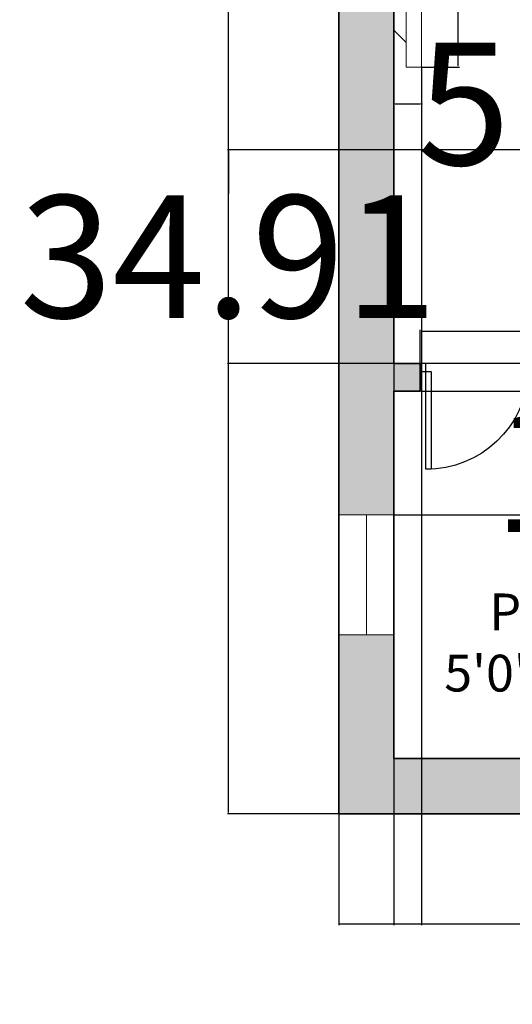
# Model space of a CAD drawing. Units: inches. Extents: x 305 to 776, y 38 to 479.
# Tile 1 of 14: x 339 to 419, y 38 to 199. Entities that reach past the tile are written whole.
import ezdxf

# ---------------------------------------------------------------- set-up
doc = ezdxf.new("R2010")
doc.units = ezdxf.units.IN
doc.header["$MEASUREMENT"] = 0
for name, color, linetype, lineweight in [('A-ANNO-DIMS', 2, 'Continuous', 18), ('A-AREA-IDEN', 7, 'Continuous', 18), ('A-DOOR', 4, 'Continuous', 25), ('A-EQPM', 8, 'Continuous', 18), ('A-GLAZ', 4, 'Continuous', 20), ('A-WALL', 7, 'Continuous', 35), ('A-WALL-PATT', 252, 'Continuous', 13)]:
    doc.layers.add(name, color=color, linetype=linetype, lineweight=lineweight)
doc.styles.get("Standard").update_dxf_attribs({"font": 'arial.ttf'})
doc.dimstyles.get("Standard").update_dxf_attribs({"dimtxt": 20, "dimasz": 0.18, "dimexe": 0.18, "dimexo": 0.0625, "dimgap": 0.09, "dimtad": 0, "dimtih": 1, "dimtoh": 1, "dimdec": 4, "dimzin": 0, "dimdsep": 46, "dimtxsty": 'Standard', "dimcen": 0.09, "dimadec": 0, "dimazin": 0, "dimtfac": 1, "dimtdec": 4, "dimtofl": 0, "dimtmove": 0, "dimatfit": 3, "dimfxl": 1, "dimtolj": 1, "dimtzin": 0, "dimarcsym": 0})

# ---------------------------------------------------------------- blocks, each defined once
blk = doc.blocks.new('W1')
blk.add_line((867.01, 338.44), (847.41, 338.44))
blk.add_lwpolyline([(847.41, 333.94), (867.01, 333.94), (867.01, 342.94), (847.41, 342.94)], close=True)
blk = doc.blocks.new('TV')
for p, q in [((722.63, 295.63), (720.13, 295.63)), ((720.13, 295.63), (720.13, 255.63)), ((722.63, 255.63), (722.63, 295.63)), ((720.13, 291.63), (718.13, 289.63)), ((718.13, 289.63), (718.13, 261.63)), ((720.13, 259.63), (718.13, 261.63)), ((720.13, 255.63), (722.63, 255.63))]:
    blk.add_line(p, q)
blk = doc.blocks.new('A$C16FA5A5B')
for p, q in [((50, 487.5), (25, 487.5)), ((25, 487.5), (25, 37.5)), ((50, 37.5), (50, 487.5)), ((950, 37.5), (950, 487.5)), ((950, 487.5), (975, 487.5)), ((975, 487.5), (975, 37.5)), ((0, 0), (0, 37.5)), ((0, 37.5), (25, 37.5)), ((25, 0), (0, 0)), ((25, 37.5), (25, 0)), ((25, 37.5), (50, 37.5)), ((975, 37.5), (950, 37.5)), ((975, 37.5), (975, 0)), ((1000, 37.5), (975, 37.5)), ((975, 0), (1000, 0)), ((1000, 0), (1000, 37.5))]:
    blk.add_line(p, q)
for centre, start, end in [((28.6, 15.6), 2.662, 90.4344), ((971.4, 15.6), 89.5656, 177.338)]:
    blk.add_arc(centre, 471.9, start, end)
blk = doc.blocks.new('*D21')
at = {"layer": 'A-ANNO-DIMS', "color": 0, "lineweight": -2, "transparency": 16777216}
for p, q in [((403.93, 142.94), (403.93, 148.37)), ((404.11, 148.19), (439.15, 148.19)), ((439.33, 142.94), (439.33, 148.37)), ((439.33, 148.19), (439.51, 148.19))]:
    blk.add_line(p, q, dxfattribs=at)
at = {"layer": 'A-ANNO-DIMS', "color": 0, "transparency": 16777216}
for points in [[(404.11, 148.22), (404.11, 148.16), (403.93, 148.19)], [(439.15, 148.22), (439.15, 148.16), (439.33, 148.19)]]:
    blk.add_solid(points, dxfattribs=at)
at = {"layer": 'Defpoints', "color": 0, "transparency": 16777216}
for p in [(439.33, 148.19), (403.93, 142.88), (439.33, 142.88)]:
    blk.add_point(p, dxfattribs=at)
at = {"layer": 'A-ANNO-DIMS', "color": 0, "transparency": 16777216, "insert": (560.63, 148.19), "char_height": 20, "attachment_point": 5}
blk.add_mtext('\\A1;DOUBLE DOOR 35', dxfattribs=at)
blk = doc.blocks.new('*D22')
at = {"layer": 'A-ANNO-DIMS', "color": 0, "lineweight": -2, "transparency": 16777216}
for p, q in [((439.4, 142.88), (444.82, 142.88)), ((444.64, 142.7), (444.64, 125.74)), ((439.4, 125.56), (444.82, 125.56)), ((444.64, 125.56), (444.64, 125.38)), ((444.64, 125.38), (444.46, 125.38))]:
    blk.add_line(p, q, dxfattribs=at)
at = {"layer": 'A-ANNO-DIMS', "color": 0, "transparency": 16777216}
for points in [[(444.61, 142.7), (444.67, 142.7), (444.64, 142.88)], [(444.61, 125.74), (444.67, 125.74), (444.64, 125.56)]]:
    blk.add_solid(points, dxfattribs=at)
at = {"layer": 'Defpoints', "color": 0, "transparency": 16777216}
for p in [(439.33, 142.88), (439.33, 125.56), (444.64, 125.56)]:
    blk.add_point(p, dxfattribs=at)
at = {"layer": 'A-ANNO-DIMS', "color": 0, "transparency": 16777216, "insert": (430.99, 125.38), "char_height": 20, "attachment_point": 5}
blk.add_mtext('\\A1;17', dxfattribs=at)
blk = doc.blocks.new('*D37')
at = {"layer": 'A-ANNO-DIMS', "color": 0, "lineweight": -2, "transparency": 16777216}
for p, q in [((476.35, 237.03), (483.22, 237.03)), ((483.04, 236.85), (483.04, 224.94)), ((483.04, 192.15), (483.04, 204.06)), ((476.35, 191.97), (483.22, 191.97))]:
    blk.add_line(p, q, dxfattribs=at)
at = {"layer": 'A-ANNO-DIMS', "color": 0, "transparency": 16777216}
for points in [[(483.01, 236.85), (483.07, 236.85), (483.04, 237.03)], [(483.01, 192.15), (483.07, 192.15), (483.04, 191.97)]]:
    blk.add_solid(points, dxfattribs=at)
at = {"layer": 'Defpoints', "color": 0, "transparency": 16777216}
for p in [(476.28, 237.03), (483.04, 237.03), (476.28, 191.97)]:
    blk.add_point(p, dxfattribs=at)
at = {"layer": 'A-ANNO-DIMS', "color": 0, "transparency": 16777216, "insert": (483.04, 214.5), "char_height": 20, "attachment_point": 5}
blk.add_mtext('\\A1;COFFEE TABLE 45', dxfattribs=at)
blk = doc.blocks.new('*D39')
at = {"layer": 'A-ANNO-DIMS', "color": 0, "lineweight": -2, "transparency": 16777216}
for p, q in [((404.2, 231.29), (410.31, 231.29)), ((410.13, 231.11), (410.13, 221.59)), ((410.13, 191.47), (410.13, 200.99)), ((404.2, 191.29), (410.31, 191.29))]:
    blk.add_line(p, q, dxfattribs=at)
at = {"layer": 'A-ANNO-DIMS', "color": 0, "transparency": 16777216}
for points in [[(410.1, 231.11), (410.16, 231.11), (410.13, 231.29)], [(410.1, 191.47), (410.16, 191.47), (410.13, 191.29)]]:
    blk.add_solid(points, dxfattribs=at)
at = {"layer": 'Defpoints', "color": 0, "transparency": 16777216}
for p in [(404.13, 231.29), (410.13, 231.29), (404.13, 191.29)]:
    blk.add_point(p, dxfattribs=at)
at = {"layer": 'A-ANNO-DIMS', "color": 0, "transparency": 16777216, "insert": (410.13, 211.29), "char_height": 20, "attachment_point": 5}
blk.add_mtext('\\A1;TV 40', dxfattribs=at)
blk = doc.blocks.new('*D40')
at = {"layer": 'A-ANNO-DIMS', "color": 0, "lineweight": -2, "transparency": 16777216}
for p, q in [((399.63, 191.23), (399.63, 185.11)), ((404.13, 191.23), (404.13, 185.11)), ((399.81, 185.29), (403.95, 185.29)), ((404.13, 185.29), (404.31, 185.29))]:
    blk.add_line(p, q, dxfattribs=at)
at = {"layer": 'A-ANNO-DIMS', "color": 0, "transparency": 16777216}
for points in [[(399.81, 185.32), (399.81, 185.26), (399.63, 185.29)], [(403.95, 185.32), (403.95, 185.26), (404.13, 185.29)]]:
    blk.add_solid(points, dxfattribs=at)
at = {"layer": 'Defpoints', "color": 0, "transparency": 16777216}
for p in [(399.63, 191.29), (404.13, 191.29), (404.13, 185.29)]:
    blk.add_point(p, dxfattribs=at)
at = {"layer": 'A-ANNO-DIMS', "color": 0, "transparency": 16777216, "insert": (411.03, 185.29), "char_height": 20, "attachment_point": 5}
blk.add_mtext('\\A1;5', dxfattribs=at)
blk = doc.blocks.new('*D45')
at = {"layer": 'A-ANNO-DIMS', "color": 0, "lineweight": -2, "transparency": 16777216}
for p, q in [((390.63, 69.32), (390.63, 51.2)), ((630.63, 69.32), (630.63, 51.2)), ((390.81, 51.38), (488.31, 51.38)), ((630.45, 51.38), (532.95, 51.38))]:
    blk.add_line(p, q, dxfattribs=at)
at = {"layer": 'A-ANNO-DIMS', "color": 0, "transparency": 16777216}
for points in [[(390.81, 51.41), (390.81, 51.35), (390.63, 51.38)], [(630.45, 51.41), (630.45, 51.35), (630.63, 51.38)]]:
    blk.add_solid(points, dxfattribs=at)
at = {"layer": 'Defpoints', "color": 0, "transparency": 16777216}
for p in [(390.63, 69.38), (630.63, 69.38), (630.63, 51.38)]:
    blk.add_point(p, dxfattribs=at)
at = {"layer": 'A-ANNO-DIMS', "color": 0, "transparency": 16777216, "insert": (510.63, 51.38), "char_height": 20, "attachment_point": 5}
blk.add_mtext('\\A1;240', dxfattribs=at)
blk = doc.blocks.new('*D46')
at = {"layer": 'A-ANNO-DIMS', "color": 0, "lineweight": -2, "transparency": 16777216}
for p, q in [((390.57, 429.38), (372.45, 429.38)), ((372.63, 429.2), (372.63, 259.69)), ((372.63, 69.56), (372.63, 239.07)), ((390.57, 69.38), (372.45, 69.38))]:
    blk.add_line(p, q, dxfattribs=at)
at = {"layer": 'A-ANNO-DIMS', "color": 0, "transparency": 16777216}
for points in [[(372.6, 429.2), (372.66, 429.2), (372.63, 429.38)], [(372.6, 69.56), (372.66, 69.56), (372.63, 69.38)]]:
    blk.add_solid(points, dxfattribs=at)
at = {"layer": 'Defpoints', "color": 0, "transparency": 16777216}
for p in [(372.63, 429.38), (390.63, 429.38), (390.63, 69.38)]:
    blk.add_point(p, dxfattribs=at)
at = {"layer": 'A-ANNO-DIMS', "color": 0, "transparency": 16777216, "insert": (372.63, 249.38), "char_height": 20, "attachment_point": 5}
blk.add_mtext('\\A1;360', dxfattribs=at)
blk = doc.blocks.new('*D48')
at = {"layer": 'A-ANNO-DIMS', "color": 0, "lineweight": -2, "transparency": 16777216}
for p, q in [((404, 138.38), (648.81, 138.38)), ((648.63, 138.38), (648.63, 138.56)), ((648.63, 138.56), (648.81, 138.56)), ((648.63, 118.36), (648.63, 138.2)), ((399.7, 118.18), (648.81, 118.18))]:
    blk.add_line(p, q, dxfattribs=at)
at = {"layer": 'A-ANNO-DIMS', "color": 0, "transparency": 16777216}
for points in [[(648.6, 138.2), (648.66, 138.2), (648.63, 138.38)], [(648.6, 118.36), (648.66, 118.36), (648.63, 118.18)]]:
    blk.add_solid(points, dxfattribs=at)
at = {"layer": 'Defpoints', "color": 0, "transparency": 16777216}
for p in [(403.93, 138.38), (648.63, 138.38), (399.63, 118.18)]:
    blk.add_point(p, dxfattribs=at)
at = {"layer": 'A-ANNO-DIMS', "color": 0, "transparency": 16777216, "insert": (674.95, 138.56), "char_height": 20, "attachment_point": 5}
blk.add_mtext('\\A1;20.2', dxfattribs=at)
blk = doc.blocks.new('*D62')
at = {"layer": 'A-ANNO-DIMS', "color": 0, "lineweight": -2, "transparency": 16777216}
for p, q in [((399.63, 336.32), (399.63, 51.2)), ((423.23, 336.32), (423.23, 51.2)), ((399.81, 51.38), (423.05, 51.38)), ((423.23, 51.38), (423.41, 51.38))]:
    blk.add_line(p, q, dxfattribs=at)
at = {"layer": 'A-ANNO-DIMS', "color": 0, "transparency": 16777216}
for points in [[(399.81, 51.41), (399.81, 51.35), (399.63, 51.38)], [(423.05, 51.41), (423.05, 51.35), (423.23, 51.38)]]:
    blk.add_solid(points, dxfattribs=at)
at = {"layer": 'Defpoints', "color": 0, "transparency": 16777216}
for p in [(399.63, 336.38), (423.23, 336.38), (423.23, 51.38)]:
    blk.add_point(p, dxfattribs=at)
at = {"layer": 'A-ANNO-DIMS', "color": 0, "transparency": 16777216, "insert": (449.64, 51.38), "char_height": 20, "attachment_point": 5}
blk.add_mtext('\\A1;23.6', dxfattribs=at)
blk = doc.blocks.new('*D65')
at = {"layer": 'A-ANNO-DIMS', "color": 0, "lineweight": -2, "transparency": 16777216}
for p, q in [((399.63, 351.22), (399.63, 51.2)), ((421.89, 351.22), (421.89, 51.2)), ((399.81, 51.38), (421.71, 51.38)), ((421.89, 51.38), (422.07, 51.38))]:
    blk.add_line(p, q, dxfattribs=at)
at = {"layer": 'A-ANNO-DIMS', "color": 0, "transparency": 16777216}
for points in [[(399.81, 51.41), (399.81, 51.35), (399.63, 51.38)], [(421.71, 51.41), (421.71, 51.35), (421.89, 51.38)]]:
    blk.add_solid(points, dxfattribs=at)
at = {"layer": 'Defpoints', "color": 0, "transparency": 16777216}
for p in [(399.63, 351.28), (421.89, 351.28), (421.89, 51.38)]:
    blk.add_point(p, dxfattribs=at)
at = {"layer": 'A-ANNO-DIMS', "color": 0, "transparency": 16777216, "insert": (463.84, 51.38), "char_height": 20, "attachment_point": 5}
blk.add_mtext('\\A1;22.257', dxfattribs=at)
blk = doc.blocks.new('*D72')
at = {"layer": 'A-ANNO-DIMS', "color": 0, "lineweight": -2, "transparency": 16777216}
for p, q in [((446.24, 195.91), (446.24, 51.2)), ((404.13, 191.23), (404.13, 51.2)), ((404.31, 51.38), (446.06, 51.38)), ((446.24, 51.38), (446.42, 51.38))]:
    blk.add_line(p, q, dxfattribs=at)
at = {"layer": 'A-ANNO-DIMS', "color": 0, "transparency": 16777216}
for points in [[(404.31, 51.41), (404.31, 51.35), (404.13, 51.38)], [(446.06, 51.41), (446.06, 51.35), (446.24, 51.38)]]:
    blk.add_solid(points, dxfattribs=at)
at = {"layer": 'Defpoints', "color": 0, "transparency": 16777216}
for p in [(446.24, 195.97), (404.13, 191.29), (446.24, 51.38)]:
    blk.add_point(p, dxfattribs=at)
at = {"layer": 'A-ANNO-DIMS', "color": 0, "transparency": 16777216, "insert": (478.73, 51.38), "char_height": 20, "attachment_point": 5}
blk.add_mtext('\\A1;42.11', dxfattribs=at)
blk = doc.blocks.new('*D73')
at = {"layer": 'A-ANNO-DIMS', "color": 0, "lineweight": -2, "transparency": 16777216}
for p, q in [((509.31, 177.79), (372.45, 177.79)), ((372.63, 177.61), (372.63, 170.64)), ((372.63, 143.06), (372.63, 150.03)), ((476.67, 142.88), (372.45, 142.88))]:
    blk.add_line(p, q, dxfattribs=at)
at = {"layer": 'A-ANNO-DIMS', "color": 0, "transparency": 16777216}
for points in [[(372.6, 177.61), (372.66, 177.61), (372.63, 177.79)], [(372.6, 143.06), (372.66, 143.06), (372.63, 142.88)]]:
    blk.add_solid(points, dxfattribs=at)
at = {"layer": 'Defpoints', "color": 0, "transparency": 16777216}
for p in [(509.37, 177.79), (372.63, 142.88), (476.73, 142.88)]:
    blk.add_point(p, dxfattribs=at)
at = {"layer": 'A-ANNO-DIMS', "color": 0, "transparency": 16777216, "insert": (372.63, 160.34), "char_height": 20, "attachment_point": 5}
blk.add_mtext('\\A1;34.91', dxfattribs=at)

msp = doc.modelspace()

# ---------------------------------------------------------------- hatches: boundary and pattern name
at = {"layer": 'A-WALL-PATT'}
h = msp.add_hatch(color=256, dxfattribs=at)
h.dxf.hatch_style = 1
h.paths.add_polyline_path([(481.3329, 429.382), (390.6329, 429.382), (390.6329, 398.067), (399.6329, 398.067), (399.6329, 420.382), (465.6329, 420.382), (465.6329, 331.882), (470.1329, 331.882), (470.1329, 355.882), (512.1329, 355.882), (512.1329, 337.282), (512.1329, 337.282), (515.8592, 337.282), (516.6329, 337.282), (516.6329, 360.382), (513.3171, 360.382), (470.1329, 360.382), (470.1329, 420.382), (481.3329, 420.382)])
h.paths.add_polyline_path([(630.6329, 429.382), (500.9329, 429.382), (500.9329, 420.382), (502.8693, 420.382), (512.1329, 420.382), (512.1329, 391.882), (516.6329, 391.882), (516.6329, 420.382), (621.6329, 420.382), (621.6329, 388.182), (630.6329, 388.182)])
h.paths.add_polyline_path([(630.6329, 329.382), (621.6329, 329.382), (621.6329, 301.882), (512.1329, 301.882), (512.1329, 297.382), (515.8592, 297.382), (557.6329, 297.382), (621.6329, 297.382), (621.6329, 286.182), (630.6329, 286.182)])
h.paths.add_polyline_path([(630.6329, 266.582), (621.6329, 266.582), (621.6329, 255.382), (589.1329, 255.382), (589.1329, 250.882), (621.6329, 250.882), (621.6329, 226.282), (630.6329, 226.282)])
h.paths.add_polyline_path([(630.6329, 167.482), (621.6329, 167.482), (621.6329, 149.1444), (621.6329, 142.882), (516.6329, 142.882), (516.6329, 261.982), (512.1329, 261.982), (512.1329, 138.382), (621.6329, 138.382), (621.6329, 78.382), (512.1329, 78.382), (512.1329, 69.382), (630.6329, 69.382)])
h.paths.add_polyline_path([(464.1329, 138.382), (476.7329, 138.382), (476.7329, 142.1084), (476.7329, 142.882), (459.6329, 142.882), (459.6329, 78.382), (399.6329, 78.382), (399.6329, 98.582), (390.6329, 98.582), (390.6329, 69.382), (464.1329, 69.382)])
h.paths.add_polyline_path([(459.6329, 142.882), (439.3329, 142.882), (439.3329, 138.382), (459.6329, 138.382)], flags=17)
h.paths.add_polyline_path([(399.6329, 138.382), (403.9329, 138.382), (403.9329, 141.5545), (403.9329, 141.5545), (403.9329, 142.882), (399.6329, 142.882), (399.6329, 250.4819), (390.6329, 250.4819), (390.6329, 118.182), (399.6329, 118.182)])
h.paths.add_polyline_path([(399.6329, 331.882), (428.2629, 331.882), (428.2629, 336.382), (399.6329, 336.382), (399.6329, 358.697), (390.6329, 358.697), (390.6329, 309.2819), (399.6329, 309.2819)])

# ---------------------------------------------------------------- linework, layer by layer
at = {"layer": 'A-WALL'}
for p, q in [((399.6329, 331.882), (399.6329, 142.882)), ((403.9329, 142.882), (399.6329, 142.882)), ((403.9329, 138.382), (403.9329, 142.882)), ((399.6329, 138.382), (399.6329, 78.382)), ((399.6329, 138.382), (403.9329, 138.382)), ((403.9329, 138.382), (399.6329, 138.382)), ((399.6329, 78.382), (459.6329, 78.382))]:
    msp.add_line(p, q, dxfattribs=at)
msp.add_lwpolyline([(390.6329, 69.382), (630.6329, 69.382), (630.6329, 429.382), (390.6329, 429.382)], close=True, dxfattribs=at)

# ---------------------------------------------------------------- block references
at = {"layer": 'A-DOOR', "xscale": -0.0354, "yscale": 0.0354, "zscale": 0.0354, "rotation": 180}
msp.add_blockref('A$C16FA5A5B', (403.9329, 142.882), dxfattribs=at)
at = {"layer": 'A-EQPM'}
msp.add_blockref('TV', (-318.4969, -64.3429), dxfattribs=at)
at = {"layer": 'A-GLAZ', "rotation": 90}
msp.add_blockref('W1', (733.5758, -748.8301), dxfattribs=at)

# ---------------------------------------------------------------- texts
at = {"layer": 'A-AREA-IDEN', "insert": (386.3367, 105.3331), "char_height": 6, "attachment_point": 1}
msp.add_mtext_dynamic_manual_height_columns('\\pxqc;PUJA\\P5\'0"X5\'0"', width=78.185, gutter_width=1, heights=[0], dxfattribs=at)

# ---------------------------------------------------------------- dimensions: what is measured, and where the dimension line sits
at = {"layer": 'A-ANNO-DIMS'}
for base, p1, p2, angle, override, picture, middle in [((372.6314, 429.382), (390.6329, 69.382), (390.6329, 429.382), 90, {"dimdec": 0, "dimlfac": 1, "dimrnd": 0, "dimzin": 0, "dimdsep": 46, "dimlunit": 2}, '*D46', (372.6314, 249.382)), ((372.6314, 142.882), (509.3694, 177.7903), (476.7329, 142.882), 90, {"dimdec": 2, "dimlfac": 1, "dimrnd": 0, "dimzin": 0, "dimdsep": 46, "dimlunit": 2}, '*D73', (372.6314, 160.3362)), ((648.6344, 138.382), (399.6329, 118.182), (403.9329, 138.382), 90, {"dimdec": 1, "dimlfac": 1, "dimrnd": 0, "dimzin": 0, "dimdsep": 46, "dimlunit": 2}, '*D48', (674.9481, 138.562)), ((444.6429, 125.5565), (439.3329, 142.882), (439.3329, 125.5565), 270, {"dimdec": 0, "dimlfac": 1, "dimrnd": 0, "dimzin": 0, "dimdsep": 46, "dimlunit": 2}, '*D22', (430.9895, 125.3765))]:
    dim = msp.add_linear_dim(base=base, p1=p1, p2=p2, angle=angle, dimstyle='Standard', override=override, dxfattribs=at)
    dim.commit()
    dim.dimension.update_dxf_attribs({"geometry": picture, "text_midpoint": middle})
for base, p1, p2, override, picture, middle in [((421.8895, 51.3805), (399.6329, 351.2815), (421.8895, 351.2815), {"dimdec": 3, "dimlfac": 1, "dimrnd": 0, "dimzin": 0, "dimdsep": 46, "dimlunit": 2}, '*D65', (463.8444, 51.3805)), ((423.2329, 51.3805), (399.6329, 336.382), (423.2329, 336.382), {"dimdec": 1, "dimlfac": 1, "dimrnd": 0, "dimzin": 0, "dimdsep": 46, "dimlunit": 2}, '*D62', (449.6421, 51.3805)), ((404.1329062952, 185.2915214337), (399.6329062952, 191.2915214337), (404.1329062952, 191.2915214337), {"dimdec": 0, "dimlfac": 1, "dimrnd": 0, "dimzin": 0, "dimdsep": 46, "dimlunit": 2}, '*D40', (411.0331927891, 185.2915214337)), ((446.2445, 51.3805), (404.1329, 191.2915), (446.2445, 195.9726), {"dimdec": 2, "dimlfac": 1, "dimrnd": 0, "dimzin": 0, "dimdsep": 46, "dimlunit": 2}, '*D72', (478.7314, 51.3805)), ((630.6329, 51.3805), (390.6329, 69.382), (630.6329, 69.382), {"dimdec": 0, "dimlfac": 1, "dimrnd": 0, "dimzin": 0, "dimdsep": 46, "dimlunit": 2}, '*D45', (510.6329, 51.3805))]:
    dim = msp.add_linear_dim(base=base, p1=p1, p2=p2, dimstyle='Standard', override=override, dxfattribs=at)
    dim.commit()
    dim.dimension.update_dxf_attribs({"geometry": picture, "text_midpoint": middle})
for base, p1, p2, text, picture, middle in [((483.0416, 237.0288), (476.2832, 191.9726), (476.2832, 237.0288), 'COFFEE TABLE <>', '*D37', (483.0416, 214.5007)), ((410.1329, 231.2915), (404.1329, 191.2915), (404.1329, 231.2915), 'TV <>', '*D39', (410.1329, 211.2915))]:
    dim = msp.add_linear_dim(base=base, p1=p1, p2=p2, angle=90, text=text, dimstyle='Standard', override={"dimdec": 0, "dimlfac": 1, "dimrnd": 0, "dimzin": 0, "dimdsep": 46, "dimlunit": 2}, dxfattribs=at)
    dim.commit()
    dim.dimension.update_dxf_attribs({"geometry": picture, "text_midpoint": middle})
dim = msp.add_linear_dim(base=(439.3329, 148.192), p1=(403.9329, 142.882), p2=(439.3329, 142.882), text='DOUBLE DOOR <>', dimstyle='Standard', override={"dimdec": 0, "dimlfac": 1, "dimrnd": 0, "dimzin": 0, "dimdsep": 46, "dimlunit": 2}, dxfattribs=at)
dim.commit()
dim.dimension.update_dxf_attribs({"geometry": '*D21', "text_midpoint": (560.6261, 148.192)})

doc.saveas('drawing.dxf')
